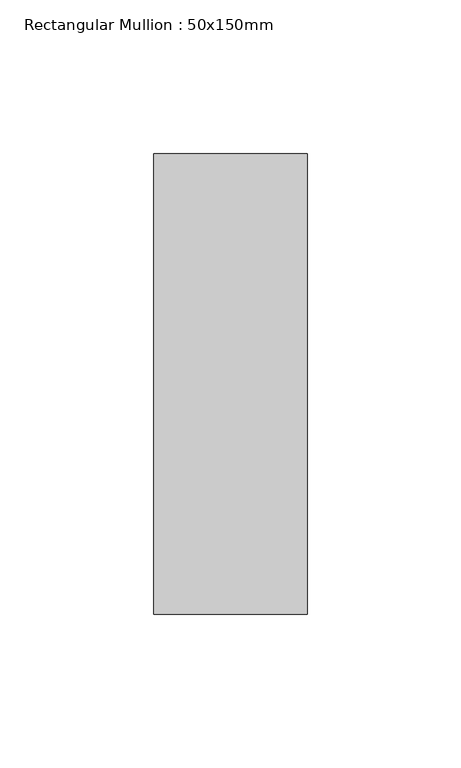
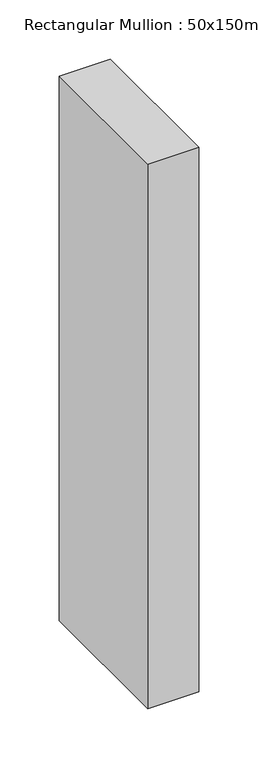
"""IFC4 building model written with IfcOpenShell, lengths in millimetres: member geometry, Rectangular Mullion : 50x150mm."""

from ifc_helpers import new_model, si_unit, frame, origin, place, context, project, spatial, polyline, outline, extrude, source, transform, mapped, element, save


def rectangular_mullion_50x150mm_61ade493(model_context):
    return source(origin(), model_context, "Body", "SweptSolid", [
        extrude(outline(polyline([(0.0, 75.0), (0.0, -75.0), (-50.0, -75.0), (-50.0, 75.0), (0.0, 75.0)])), frame((0.0, 0.0, -563.0333333), z_axis=(0.0, 0.0, 1.0), x_axis=(1.0, 0.0, 0.0)), (0.0, 0.0, 1.0), 563.0333333),
    ])


if __name__ == "__main__":
    model = new_model("IFC4")
    model_context = context("Model", 3, world=origin())
    ifc_project = project(units=[si_unit("LENGTHUNIT", "METRE", prefix="MILLI")], contexts=[model_context])
    site = spatial("IfcSite", under=ifc_project)
    building = spatial("IfcBuilding", under=site)
    placement = place(None, origin())
    rectangular_mullion_50x150mm_shape = rectangular_mullion_50x150mm_61ade493(model_context)
    element("IfcMember", 1, ObjectType="Rectangular Mullion : 50x150mm", at=placement, inside=building, context=model_context, shape_type="MappedRepresentation", body=[
        mapped(rectangular_mullion_50x150mm_shape, transform((0.0, 0.0, 0.0), x_axis=(1.0, 0.0, 0.0), y_axis=(0.0, 1.0, 0.0), z_axis=(0.0, 0.0, 1.0))),
    ])
    save(model, "model.ifc")

# Revit data of these elements
# Type "Rectangular Mullion : 50x150mm"
#   Keynote = "H11"
#   built-in parameter 1007304 = 0.492126 (stored number, unit not read)
#   built-in parameter 1007301 = 0.082021 (stored number, unit not read)
#   built-in parameter 1007300 = 0.082021 (stored number, unit not read)
# Element 1 (IfcMember, "Rectangular Mullion : 50x150mm")
#   Materials on its faces: "Aluminium"
# Materials
#   "Aluminium": class "Metal", colour RGB 247 247 247, transparency 0, Description = "Aluminium 6061", Cost = 0
